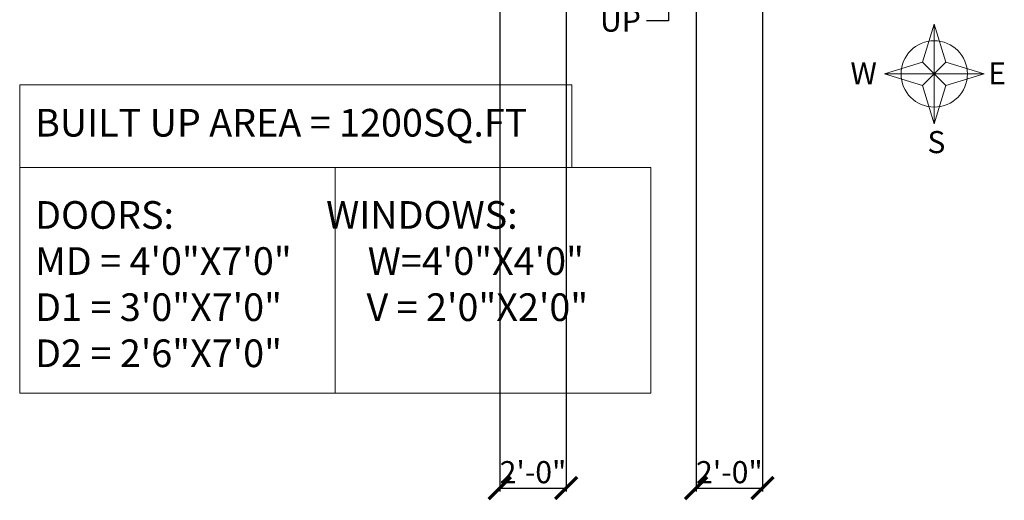
# Model space of a CAD drawing. Units: inches. Extents: x 21865 to 22885, y 36660 to 37408.
# Tile 1 of 6: x 21916 to 22272, y 36660 to 36833. Entities that reach past the tile are written whole.
import ezdxf
from ezdxf import colors
from ezdxf.entities.mleader import LeaderData, LeaderLine
from ezdxf.math import Vec2, Vec3

# ---------------------------------------------------------------- set-up
doc = ezdxf.new("R2010")
doc.units = ezdxf.units.IN
for name, color, linetype, lineweight in [('A-ANNO-DIMS', 2, 'Continuous', 18), ('A-ANNO-SYMB', 7, 'Continuous', 18), ('A-ANNO-TEXT', 7, 'Continuous', 18)]:
    doc.layers.add(name, color=color, linetype=linetype, lineweight=lineweight)
doc.layers.add('A-ANNO-SCHD', color=254, linetype='Continuous', lineweight=18, true_color=0xddb3d4)
doc.styles.get("Standard").update_dxf_attribs({"font": 'arial.ttf'})
doc.dimstyles.new('ISO-25', dxfattribs={"dimtxt": 8, "dimasz": 8, "dimexe": 1.25, "dimexo": 0.625, "dimtad": 1, "dimlunit": 3, "dimtxsty": 'Standard', "dimblk": 'ARCHTICK', "dimcen": 2.5, "dimclrd": 4, "dimclre": 5, "dimclrt": 1, "dimadec": 0, "dimazin": 0, "dimtfac": 1, "dimtmove": 0, "dimatfit": 3, "dimfxl": 1, "dimarcsym": 0})

# ---------------------------------------------------------------- blocks, each defined once
blk = doc.blocks.new('_ArchTick')
at = {"color": 0, "linetype": 'ByBlock', "const_width": 0.15}
blk.add_lwpolyline([(-0.5, -0.5), (0.5, 0.5)], dxfattribs=at)
blk = doc.blocks.new('*D58')
at = {"layer": 'A-ANNO-DIMS', "color": 5, "lineweight": -2, "transparency": 16777216}
for p, q in [((22160.43, 37233.31), (22160.43, 36662.83)), ((22184.43, 37233.31), (22184.43, 36662.83))]:
    blk.add_line(p, q, dxfattribs=at)
at = {"layer": 'A-ANNO-DIMS', "color": 4, "lineweight": -2, "transparency": 16777216}
blk.add_line((22160.43, 36664.08), (22184.43, 36664.08), dxfattribs=at)
at = {"layer": 'Defpoints', "color": 0, "transparency": 16777216}
for p in [(22160.43, 37233.93), (22184.43, 37233.93), (22184.43, 36664.08)]:
    blk.add_point(p, dxfattribs=at)
at = {"layer": 'A-ANNO-DIMS', "color": 4, "lineweight": -2, "transparency": 16777216, "xscale": 8, "yscale": 8, "zscale": 8, "rotation": 180}
blk.add_blockref('_ArchTick', (22160.43, 36664.08), dxfattribs=at)
at = {"layer": 'A-ANNO-DIMS', "color": 4, "lineweight": -2, "transparency": 16777216, "xscale": 8, "yscale": 8, "zscale": 8}
blk.add_blockref('_ArchTick', (22184.43, 36664.08), dxfattribs=at)
at = {"layer": 'A-ANNO-DIMS', "color": 1, "transparency": 16777216, "insert": (22172.43, 36668.79), "char_height": 8, "attachment_point": 5}
blk.add_mtext('2\'-0"', dxfattribs=at)
blk = doc.blocks.new('*D59')
at = {"layer": 'A-ANNO-DIMS', "color": 5, "lineweight": -2, "transparency": 16777216}
for p, q in [((22089.43, 36955.31), (22089.43, 36662.83)), ((22113.43, 36955.31), (22113.43, 36662.83))]:
    blk.add_line(p, q, dxfattribs=at)
at = {"layer": 'A-ANNO-DIMS', "color": 4, "lineweight": -2, "transparency": 16777216}
blk.add_line((22089.43, 36664.08), (22113.43, 36664.08), dxfattribs=at)
at = {"layer": 'Defpoints', "color": 0, "transparency": 16777216}
for p in [(22089.43, 36955.93), (22113.43, 36955.93), (22113.43, 36664.08)]:
    blk.add_point(p, dxfattribs=at)
at = {"layer": 'A-ANNO-DIMS', "color": 4, "lineweight": -2, "transparency": 16777216, "xscale": 8, "yscale": 8, "zscale": 8, "rotation": 180}
blk.add_blockref('_ArchTick', (22089.43, 36664.08), dxfattribs=at)
at = {"layer": 'A-ANNO-DIMS', "color": 4, "lineweight": -2, "transparency": 16777216, "xscale": 8, "yscale": 8, "zscale": 8}
blk.add_blockref('_ArchTick', (22113.43, 36664.08), dxfattribs=at)
at = {"layer": 'A-ANNO-DIMS', "color": 1, "transparency": 16777216, "insert": (22101.43, 36668.79), "char_height": 8, "attachment_point": 5}
blk.add_mtext('2\'-0"', dxfattribs=at)

msp = doc.modelspace()

# ---------------------------------------------------------------- linework, layer by layer
at = {"layer": 'A-ANNO-SCHD'}
msp.add_line((22029.941, 36698.327), (22029.941, 36779.926), dxfattribs=at)
for points in [[(21915.84, 36779.926), (22115.517, 36779.926), (22115.517, 36809.862), (21915.84, 36809.862)], [(21915.84, 36779.926), (22144.042, 36779.926), (22144.042, 36698.327), (21915.84, 36698.327)]]:
    msp.add_lwpolyline(points, close=True, dxfattribs=at)
at = {"layer": 'A-ANNO-SYMB'}
for p, q in [((22242.25, 36818.028), (22246.493, 36831.786)), ((22246.493, 36825.786), (22246.493, 36831.786)), ((22246.493, 36831.786), (22250.735, 36818.028)), ((22246.493, 36825.786), (22246.493, 36801.786)), ((22228.493, 36813.786), (22242.25, 36818.028)), ((22246.493, 36813.786), (22242.25, 36818.028)), ((22246.493, 36813.786), (22250.735, 36818.028)), ((22250.735, 36818.028), (22264.493, 36813.786)), ((22234.493, 36813.786), (22228.493, 36813.786)), ((22242.25, 36809.543), (22228.493, 36813.786)), ((22234.493, 36813.786), (22258.493, 36813.786)), ((22246.493, 36813.786), (22242.25, 36809.543)), ((22246.493, 36813.786), (22250.735, 36809.543)), ((22264.493, 36813.786), (22250.735, 36809.543)), ((22258.493, 36813.786), (22264.493, 36813.786)), ((22246.493, 36795.786), (22242.25, 36809.543)), ((22250.735, 36809.543), (22246.493, 36795.786)), ((22246.493, 36801.786), (22246.493, 36795.786))]:
    msp.add_line(p, q, dxfattribs=at)
msp.add_circle((22246.493, 36813.786), 12, dxfattribs=at)

# ---------------------------------------------------------------- texts
at = {"layer": 'A-ANNO-SYMB', "char_height": 8}
for s, insert, width, attachment_point in [('W', (22216.182, 36818.024), 18.3528, 1), ('E', (22272.435, 36818.024), 18.3528, 3), ('S', (22244.029, 36782.647), 22.941, 7)]:
    msp.add_mtext(s, dxfattribs=dict(at, insert=insert, width=width, attachment_point=attachment_point))
at = {"layer": 'A-ANNO-TEXT', "insert": (21921.413, 36801.148), "char_height": 10, "attachment_point": 1}
msp.add_mtext_dynamic_manual_height_columns('{BUILT UP AREA = 1200SQ.FT}\\P{\\PDOORS:                  WINDOWS:}\\PMD = 4\'0"X7\'0"         W=4\'0"X4\'0"\\PD1 = 3\'0"X7\'0"          V = 2\'0"X2\'0"\\PD2 = 2\'6"X7\'0"', width=251.28696, gutter_width=12.5, heights=[0], dxfattribs=at)

# ---------------------------------------------------------------- dimensions: what is measured, and where the dimension line sits
at = {"layer": 'A-ANNO-DIMS'}
for base, p1, p2, picture, middle in [((22184.43, 36664.077), (22160.43, 37233.931), (22184.43, 37233.931), '*D58', (22172.43, 36668.787)), ((22113.43, 36664.077), (22089.43, 36955.931), (22113.43, 36955.931), '*D59', (22101.43, 36668.787))]:
    dim = msp.add_linear_dim(base=base, p1=p1, p2=p2, dimstyle='ISO-25', override={"dimdec": 1, "dimlfac": 1, "dimrnd": 0, "dimzin": 1, "dimdsep": 46, "dimlunit": 4, "dimfrac": 2}, dxfattribs=at)
    dim.commit()
    dim.dimension.update_dxf_attribs({"geometry": picture, "text_midpoint": middle})

# ---------------------------------------------------------------- leaders
at = {"layer": 'A-ANNO-TEXT'}
ml = msp.add_multileader_mtext('Standard', dxfattribs=at)
ml.set_content('UP', color=256)
ml.set_leader_properties()
ml.build(insert=Vec2(0, 0))
ml.multileader.update_dxf_attribs({"arrow_head_size": 10})
ctx = ml.context
ctx.base_point, ctx.char_height, ctx.arrow_head_size, ctx.plane_origin = Vec3(22124.274, 36832.999), 8, 10, Vec3(22150.435, 36877.931)
ctx.text_align_type = 2
notes = []
notes.append((ctx, [(0, (1, 1, 0), (22150.435, 36832.999), (-1, 0), 8, [(0, [(22150.435, 36877.931)], 0, [])])]))
ctx.mtext.insert, ctx.mtext.alignment, ctx.mtext.flow_direction = Vec3(22140.435, 36837.068), 3, 5
for ctx, leaders in notes:
    for number, flags, end, landing, length, lines in leaders:
        leader = LeaderData()
        leader.index, (leader.has_last_leader_line, leader.has_dogleg_vector, leader.attachment_direction) = number, flags
        leader.last_leader_point, leader.dogleg_vector, leader.dogleg_length = Vec3(end), Vec3(landing), length
        for number, points, colour, breaks in lines:
            line = LeaderLine()
            line.index, line.vertices, line.color, line.breaks = number, Vec3.list(points), colors.encode_raw_color(colour), breaks
            leader.lines.append(line)
        ctx.leaders.append(leader)

doc.saveas('drawing.dxf')
